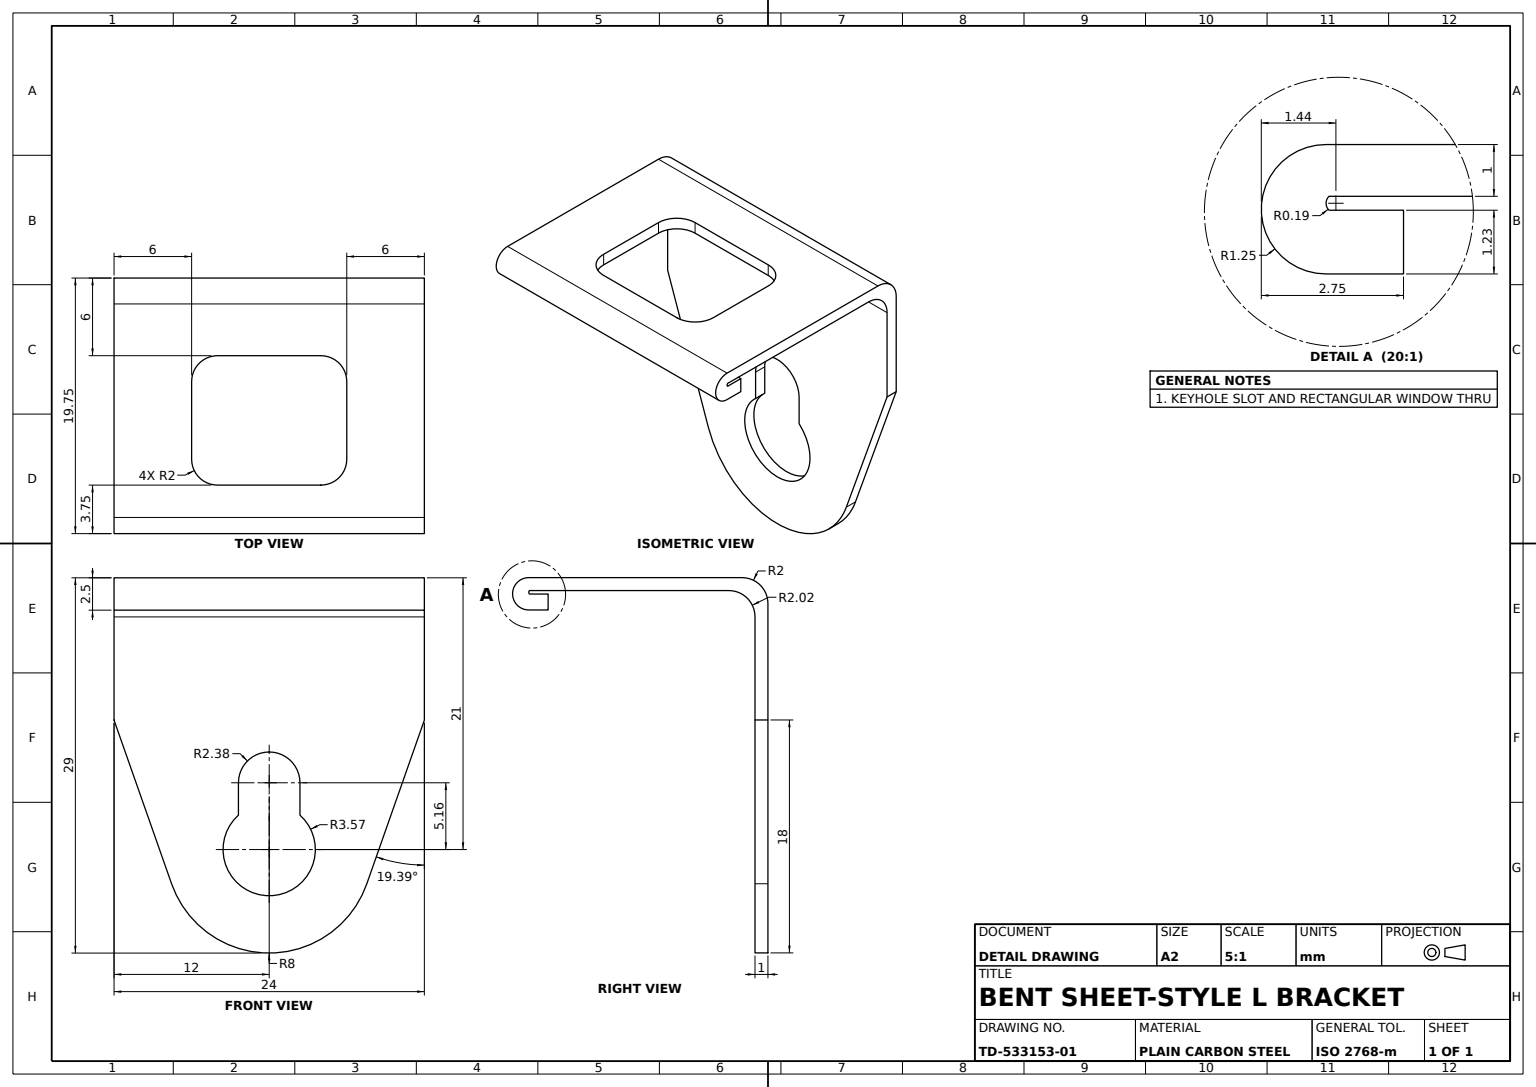
from build123d import *

# Parameters (mm, degrees)
BRACKET_BODY_DEPTH           = 12
RECTANGULAR_WINDOW_CUT_DEPTH = 5
KEYHOLE_SLOT_CUT_DEPTH       = 10
EDGE_NOTCH_CUT_DEPTH         = 2


with BuildPart() as part:
    # Bracket Profile Sketch → Bracket Body (new, symmetric)
    with BuildSketch(Plane.XY):
        with BuildLine():
            Line((2, 0), (18.5, 0))
            ThreePointArc((18.5, 0), (19.75, -1.25), (18.5, -2.5))
            Line((18.5, -2.5), (17, -2.5))
            Line((17, -2.5), (17, -1.268700577))
            Line((17, -1.268700577), (18.441553142, -1.268700577))
            ThreePointArc((18.441553142, -1.268700577), (18.497202853, -1.134350288), (18.441553142, -1))
            Line((18.441553142, -1), (3.021384942, -1))
            ThreePointArc((3.021384942, -1), (1.592049942, -1.592049942), (1, -3.021384942))
            Line((1, -3.021384942), (1, -29))
            Line((1, -29), (0, -29))
            Line((0, -29), (0, -2))
            ThreePointArc((0, -2), (0.585786438, -0.585786438), (2, 0))
        make_face()
    extrude(amount=BRACKET_BODY_DEPTH, both=True)

    # Rectangular Window Sketch → Rectangular Window Cut (cut, symmetric)
    with BuildSketch(Plane.XZ.offset(1)):
        with BuildLine():
            Line((8, -6), (14, -6))
            ThreePointArc((14, -6), (15.414213562, -5.414213562), (16, -4))
            Line((16, -4), (16, 4))
            ThreePointArc((16, 4), (15.414213562, 5.414213562), (14, 6))
            Line((14, 6), (8, 6))
            ThreePointArc((8, 6), (6.585786438, 5.414213562), (6, 4))
            Line((6, 4), (6, -4))
            ThreePointArc((6, -4), (6.585786438, -5.414213562), (8, -6))
        make_face()
    extrude(amount=RECTANGULAR_WINDOW_CUT_DEPTH, both=True, mode=Mode.SUBTRACT)

    # Keyhole Slot Sketch → Keyhole Slot Cut (cut)
    with BuildSketch(Plane(origin=(1, 0, 0), x_dir=(0, 0, -1), z_dir=(1, 0, 0))):
        with BuildLine():
            ThreePointArc((7.546363234, -23.655635881), (4.623576141, -27.52859431), (-3.9e-08, -29))
            Line((-3.9e-08, -29), (12, -29))
            Line((12, -29), (12, -11))
            Line((12, -11), (7.546363234, -23.655635881))
        make_face()
        with BuildLine():
            Line((-7.546363234, -23.655635881), (-12, -11))
            Line((-12, -11), (-12, -29))
            Line((-12, -29), (-3.9e-08, -29))
            ThreePointArc((-3.9e-08, -29), (-4.623576172, -27.528594288), (-7.546363234, -23.655635881))
        make_face()
    extrude(amount=-KEYHOLE_SLOT_CUT_DEPTH, mode=Mode.SUBTRACT)

    # Edge Notch Sketch → Edge Notch Cut (cut)
    with BuildSketch(Plane(origin=(1, 0, 0), x_dir=(0, 0, -1), z_dir=(1, 0, 0))):
        with BuildLine():
            Line((-2.38, -15.84), (-2.38, -18.339079107))
            ThreePointArc((-2.38, -18.339079107), (0, -24.57), (2.38, -18.339079107))
            Line((2.38, -18.339079107), (2.38, -15.84))
            ThreePointArc((2.38, -15.84), (0, -13.46), (-2.38, -15.84))
        make_face()
    extrude(amount=-EDGE_NOTCH_CUT_DEPTH, mode=Mode.SUBTRACT)


solid = part.part
